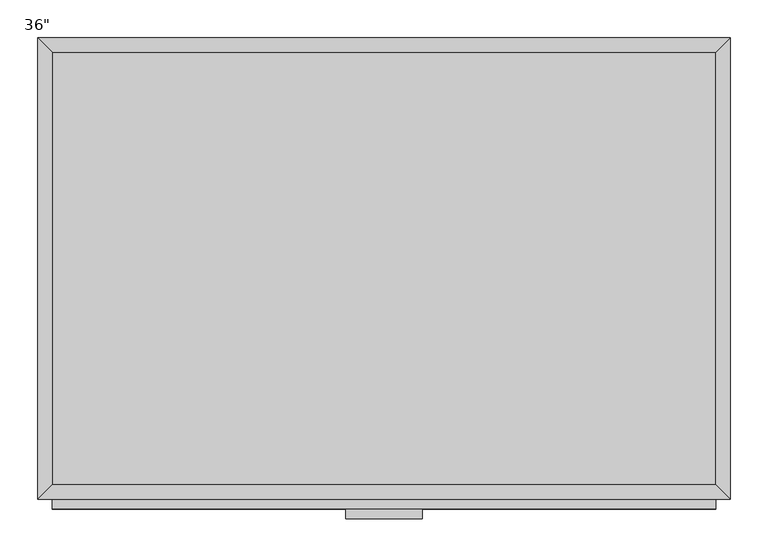
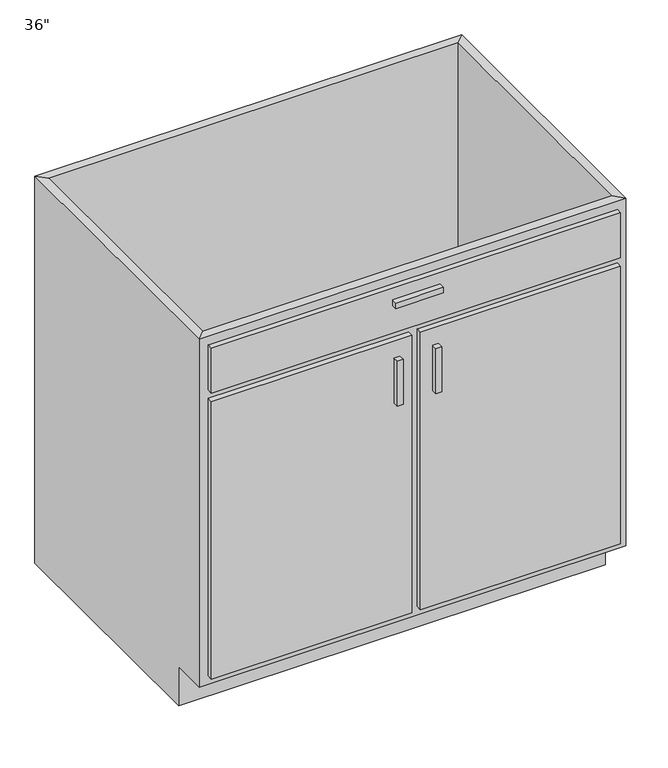
"""IFC4 building model written with IfcOpenShell, lengths in millimetres: furniture geometry."""

from ifc_helpers import new_model, si_unit, frame, origin, place, context, project, spatial, polyline, outline, extrude, faceted_brep, source, transform, mapped, element, save


def furniture_9b4ba0d7(model_context):
    return source(origin(), model_context, "Body", "SolidModel", [
        extrude(outline(polyline([(456.8877049, -19.05), (456.8877049, -590.55), (-419.4122951, -590.55), (-419.4122951, -19.05), (456.8877049, -19.05)])), frame((0.0, 0.0, 88.9), z_axis=(0.0, 0.0, 1.0), x_axis=(1.0, 0.0, 0.0)), (0.0, 0.0, 1.0), 19.05),
        faceted_brep([(-419.4122951, -533.4, 88.9), (456.8877049, -533.4, 88.9), (456.8877049, -19.05, 88.9), (-419.4122951, -19.05, 88.9), (475.9377049, 0.0, 0.0), (475.9377049, -533.4, 0.0), (-438.4622951, -533.4, 0.0), (-438.4622951, 0.0, 0.0), (-438.4622951, 0.0, 876.3), (475.9377049, 0.0, 876.3), (-438.4622951, -533.4, 88.9), (-438.4622951, -609.6, 88.9), (-438.4622951, -609.6, 876.3), (475.9377049, -533.4, 88.9), (475.9377049, -609.6, 876.3), (475.9377049, -609.6, 88.9), (456.8877049, -590.55, 876.3), (456.8877049, -590.55, 88.9), (-419.4122951, -590.55, 88.9), (-419.4122951, -590.55, 876.3), (-419.4122951, -19.05, 876.3), (456.8877049, -19.05, 876.3)], [[[0, 1, 2, 3]], [[4, 5, 6, 7]], [[4, 7, 8, 9]], [[8, 7, 6, 10, 11, 12]], [[6, 5, 13, 1, 0, 10]], [[5, 4, 9, 14, 15, 13]], [[16, 17, 18, 19]], [[16, 19, 12, 14]], [[14, 12, 11, 15]], [[18, 17, 15, 11]], [[19, 18, 0, 3, 20]], [[12, 19, 20, 8]], [[18, 11, 10, 0]], [[20, 3, 2, 21]], [[8, 20, 21, 9]], [[17, 16, 21, 2, 1]], [[16, 14, 9, 21]], [[15, 17, 1, 13]]]),
        extrude(outline(polyline([(456.8877049, -622.3), (-419.4122951, -622.3), (-419.4122951, -609.6), (456.8877049, -609.6), (456.8877049, -622.3)])), frame((0.0, 0.0, 755.65), z_axis=(0.0, 0.0, 1.0), x_axis=(1.0, 0.0, 0.0)), (0.0, 0.0, 1.0), 101.6),
        extrude(outline(polyline([(9.2127049, -622.3), (-419.4122951, -622.3), (-419.4122951, -609.6), (9.2127049, -609.6), (9.2127049, -622.3)])), frame((0.0, 0.0, 107.95), z_axis=(0.0, 0.0, 1.0), x_axis=(1.0, 0.0, 0.0)), (0.0, 0.0, 1.0), 628.65),
        extrude(outline(polyline([(456.8877049, -622.3), (28.2627049, -622.3), (28.2627049, -609.6), (456.8877049, -609.6), (456.8877049, -622.3)])), frame((0.0, 0.0, 107.95), z_axis=(0.0, 0.0, 1.0), x_axis=(1.0, 0.0, 0.0)), (0.0, 0.0, 1.0), 628.65),
        extrude(outline(polyline([(69.5377049, -635.0), (-32.0622951, -635.0), (-32.0622951, -622.3), (69.5377049, -622.3), (69.5377049, -635.0)])), frame((0.0, 0.0, 819.15), z_axis=(0.0, 0.0, 1.0), x_axis=(1.0, 0.0, 0.0)), (0.0, 0.0, 1.0), 12.7),
        extrude(outline(polyline([(-16.1872951, -635.0), (-28.8872951, -635.0), (-28.8872951, -622.3), (-16.1872951, -622.3), (-16.1872951, -635.0)])), frame((0.0, 0.0, 596.9), z_axis=(0.0, 0.0, 1.0), x_axis=(1.0, 0.0, 0.0)), (0.0, 0.0, 1.0), 101.6),
        extrude(outline(polyline([(66.3627049, -635.0), (53.6627049, -635.0), (53.6627049, -622.3), (66.3627049, -622.3), (66.3627049, -635.0)])), frame((0.0, 0.0, 596.9), z_axis=(0.0, 0.0, 1.0), x_axis=(1.0, 0.0, 0.0)), (0.0, 0.0, 1.0), 101.6),
    ])


if __name__ == "__main__":
    model = new_model("IFC4")
    model_context = context("Model", 3, world=origin())
    ifc_project = project(units=[si_unit("LENGTHUNIT", "METRE", prefix="MILLI")], contexts=[model_context])
    site = spatial("IfcSite", under=ifc_project)
    building = spatial("IfcBuilding", under=site)
    placement = place(None, origin())
    furniture_shape = furniture_9b4ba0d7(model_context)
    element("IfcFurniture", 1, ObjectType="36\"", at=placement, inside=building, context=model_context, shape_type="MappedRepresentation", body=[
        mapped(furniture_shape, transform((0.0, 0.0, 0.0), x_axis=(1.0, 0.0, 0.0), y_axis=(0.0, 1.0, 0.0), z_axis=(0.0, 0.0, 1.0))),
    ])
    save(model, "model.ifc")

# Revit data of these elements
# Type "36\""
#   Assembly Code = "C1030410"
#   Depth = 2' - 0"
#   Height = 2' - 10 1/2"
#   Toe Depth = 0' - 3"
#   Toe Height = 0' - 3 1/2"
#   Width = 3' - 0"
#   Cabinet Material = Cabinets
#   Door/Drawer Material = Cabinets
#   Handle Material = Cabinets - Handles
#   Default Elevation = 0
# Element 1 (IfcFurniture, "36\"")
#   Materials on its faces: "Cabinets", "Cabinets - Handles"
# Materials
#   "Cabinets": colour RGB 249 249 249, transparency 0
#   "Cabinets - Handles": class "Metal", colour RGB 57 57 57, transparency 0
